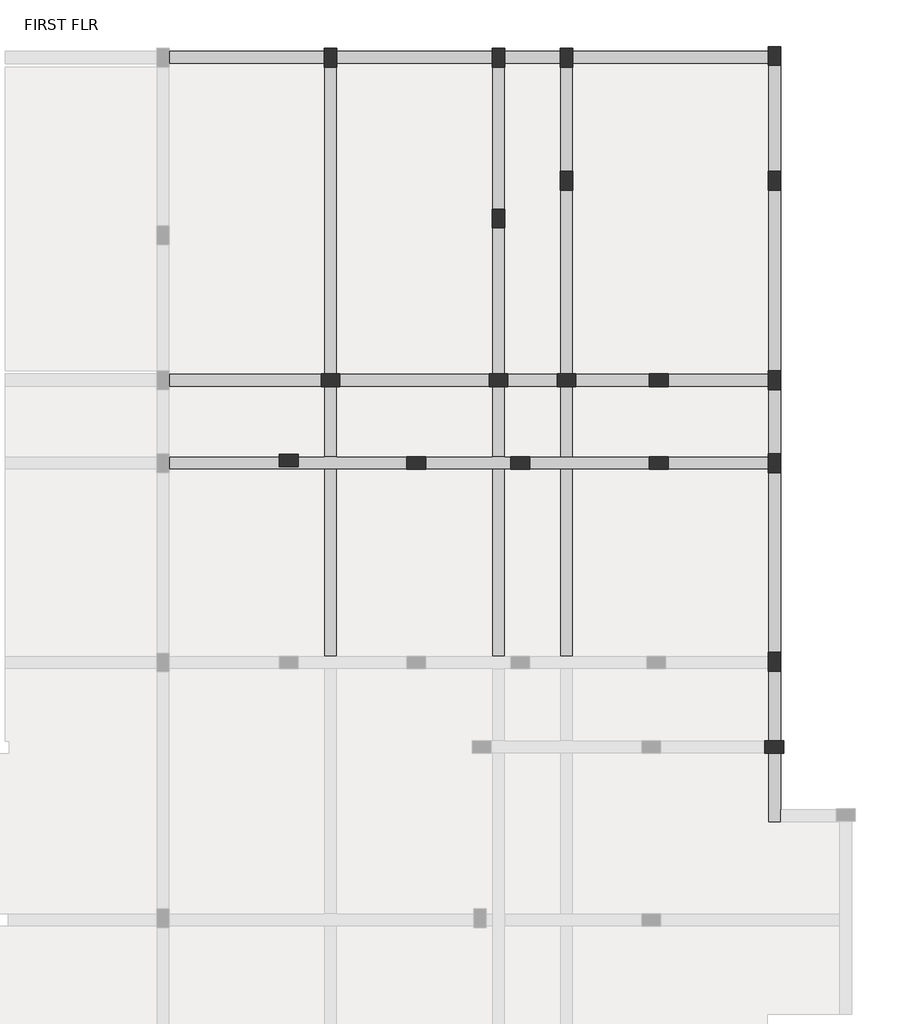
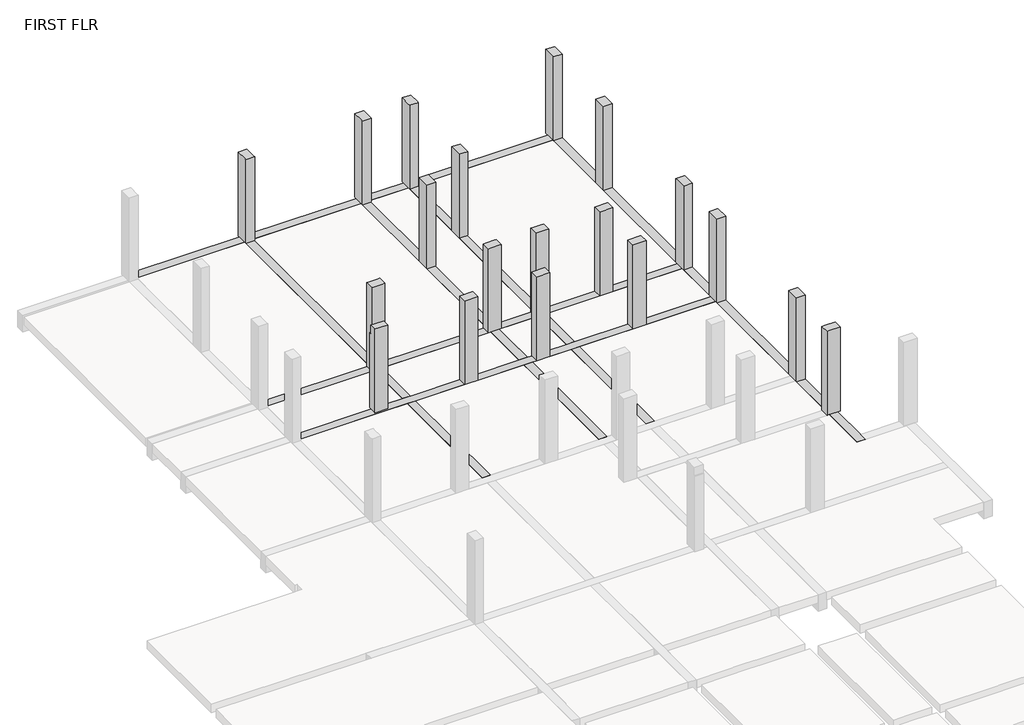
# One storey, part 5 of 5: 30 beams, 19 columns.
"""IFC4 building model written with IfcOpenShell, lengths in millimetres."""

from ifc_helpers import new_model, si_unit, frame, origin, place, context, project, spatial, polyline, outline, extrude, faceted_brep, element, save

model = new_model("IFC4")

# Units and contexts
model_context = context("Model", 3, world=origin())
ifc_project = project(units=[si_unit("LENGTHUNIT", "METRE", prefix="MILLI")], contexts=[model_context])

# Site, building, storey
site = spatial("IfcSite", under=ifc_project)
building = spatial("IfcBuilding", under=site)
storey = spatial("IfcBuildingStorey", under=building, Name="FIRST FLR", Elevation=3000.0)

# Beams
placement = place(None, origin())
element("IfcBeam", 1, ObjectType="M_Concrete-Rectangular Beam : 300 x 600mm", at=placement, inside=storey, context=model_context, shape_type="Brep", body=[
    faceted_brep([(2024.7296816, 21537.8349362, 3000.0), (2024.7296816, 21837.8349362, 3000.0), (-1671.7865686, 21837.8349362, 3000.0), (-1671.7865686, 21537.8349362, 3000.0), (2024.7296816, 21537.8349362, 2400.0), (2024.7296816, 21537.8349362, 2700.0), (-1671.7865686, 21537.8349362, 2700.0), (-1671.7865686, 21537.8349362, 2400.0), (2024.7296816, 21837.8349362, 2400.0), (-1671.7865686, 21837.8349362, 2400.0)], [[[0, 1, 2, 3]], [[4, 5, 0, 3, 6, 7]], [[8, 4, 7, 9]], [[1, 8, 9, 2]], [[2, 9, 7, 6, 3]], [[1, 0, 5, 4, 8]]]),
])
element("IfcBeam", 2, ObjectType="M_Concrete-Rectangular Beam : 300 x 600mm", at=placement, inside=storey, context=model_context, shape_type="Brep", body=[
    faceted_brep([(6032.5248054, 21537.8349362, 3000.0), (6032.5248054, 21837.8349362, 3000.0), (2324.7296816, 21837.8349362, 3000.0), (2324.7296816, 21537.8349362, 3000.0), (6032.5248054, 21537.8349362, 2400.0), (6032.5248054, 21537.8349362, 2700.0), (2324.7296816, 21537.8349362, 2700.0), (2324.7296816, 21537.8349362, 2400.0), (6032.5248054, 21837.8349362, 2400.0), (2324.7296816, 21837.8349362, 2400.0)], [[[0, 1, 2, 3]], [[4, 5, 0, 3, 6, 7]], [[8, 4, 7, 9]], [[1, 8, 9, 2]], [[2, 9, 7, 6, 3]], [[1, 0, 5, 4, 8]]]),
])
element("IfcBeam", 3, ObjectType="M_Concrete-Rectangular Beam : 300 x 600mm", at=placement, inside=storey, context=model_context, shape_type="Brep", body=[
    faceted_brep([(7656.8679014, 21537.8349362, 3000.0), (7656.8679014, 21837.8349362, 3000.0), (6332.5248054, 21837.8349362, 3000.0), (6332.5248054, 21537.8349362, 3000.0), (7656.8679014, 21537.8349362, 2400.0), (7656.8679014, 21537.8349362, 2700.0), (6332.5248054, 21537.8349362, 2700.0), (6332.5248054, 21537.8349362, 2400.0), (7656.8679014, 21837.8349362, 2400.0), (6332.5248054, 21837.8349362, 2400.0)], [[[0, 1, 2, 3]], [[4, 5, 0, 3, 6, 7]], [[8, 4, 7, 9]], [[1, 8, 9, 2]], [[2, 9, 7, 6, 3]], [[1, 0, 5, 4, 8]]]),
])
element("IfcBeam", 4, ObjectType="M_Concrete-Rectangular Beam : 300 x 600mm", at=placement, inside=storey, context=model_context, shape_type="Brep", body=[
    faceted_brep([(7956.8679014, 21837.8349362, 3000.0), (7956.8679014, 21537.8349362, 3000.0), (12619.1163908, 21537.8349362, 3000.0), (12619.1163908, 21837.8349362, 3000.0), (7956.8679014, 21537.8349362, 2700.0), (7956.8679014, 21537.8349362, 2400.0), (12619.1163908, 21537.8349362, 2400.0), (12619.1163908, 21537.8349362, 2700.0), (7956.8679014, 21837.8349362, 2400.0), (12619.1163908, 21837.8349362, 2400.0)], [[[0, 1, 2, 3]], [[1, 4, 5, 6, 7, 2]], [[5, 8, 9, 6]], [[8, 0, 3, 9]], [[0, 8, 5, 4, 1]], [[3, 2, 7, 6, 9]]]),
])
element("IfcBeam", 5, ObjectType="M_Concrete-Rectangular Beam : 300 x 600mm", at=placement, inside=storey, context=model_context, shape_type="Brep", body=[
    faceted_brep([(12916.8679014, 5087.6057249, 3000.0), (12616.8679014, 5087.6057249, 3000.0), (12616.8679014, 3435.7536525, 3000.0), (12916.8679014, 3435.7536525, 3000.0), (12916.8679014, 3735.7536525, 3000.0), (12616.8679014, 5087.6057249, 2700.0), (12616.8679014, 5087.6057249, 2400.0), (12616.8679014, 3435.7536525, 2400.0), (12616.8679014, 3435.7536525, 2700.0), (12916.8679014, 5087.6057249, 2400.0), (12916.8679014, 3735.7536525, 2400.0), (12916.8679014, 3435.7536525, 2400.0), (12916.8679014, 3435.7536525, 2700.0)], [[[0, 1, 2, 3, 4]], [[2, 1, 5, 6, 7, 8]], [[6, 9, 10, 11, 7]], [[9, 0, 4, 3, 12, 11, 10]], [[0, 9, 6, 5, 1]], [[3, 2, 8, 7, 11, 12]]]),
])
element("IfcBeam", 6, ObjectType="M_Concrete-Rectangular Beam : 300 x 600mm", at=placement, inside=storey, context=model_context, shape_type="Brep", body=[
    faceted_brep([(12616.8679014, 5387.6057249, 3000.0), (12916.8679014, 5387.6057249, 3000.0), (12916.8679014, 7044.7076276, 3000.0), (12619.1163908, 7044.7076276, 3000.0), (12619.1163908, 7399.7076276, 3000.0), (12616.8679014, 7399.7076276, 3000.0), (12616.8679014, 7099.7076276, 3000.0), (12616.8679014, 7399.7076276, 2400.0), (12616.8679014, 7099.7076276, 2400.0), (12616.8679014, 5387.6057249, 2400.0), (12616.8679014, 5387.6057249, 2700.0), (12616.8679014, 7399.7076276, 2700.0), (12916.8679014, 5387.6057249, 2400.0), (12619.1163908, 7399.7076276, 2400.0), (12619.1163908, 7044.7076276, 2400.0), (12916.8679014, 7044.7076276, 2400.0)], [[[0, 1, 2, 3, 4, 5, 6]], [[7, 8, 9, 10, 0, 6, 5, 11]], [[12, 9, 8, 7, 13, 14, 15]], [[1, 12, 15, 2]], [[1, 0, 10, 9, 12]], [[14, 3, 2, 15]], [[3, 14, 13, 4]], [[5, 4, 13, 7, 11]]]),
])
element("IfcBeam", 7, ObjectType="M_Concrete-Rectangular Beam : 300 x 600mm", at=placement, inside=storey, context=model_context, shape_type="SweptSolid", body=[
    extrude(outline(polyline([(12619.1163908, 11782.4075451), (12919.1163908, 11782.4075451), (12919.1163908, 7494.7076276), (12619.1163908, 7494.7076276), (12619.1163908, 11782.4075451)])), frame((0.0, 0.0, 2400.0), z_axis=(0.0, 0.0, 1.0), x_axis=(1.0, 0.0, 0.0)), (0.0, 0.0, 1.0), 600.0),
])
element("IfcBeam", 8, ObjectType="M_Concrete-Rectangular Beam : 300 x 600mm", at=placement, inside=storey, context=model_context, shape_type="Brep", body=[
    faceted_brep([(12619.1163908, 13762.5179708, 3000.0), (12619.1163908, 12232.4075451, 3000.0), (12919.1163908, 12232.4075451, 3000.0), (12919.1163908, 13762.5179708, 3000.0), (12919.1163908, 12232.4075451, 2400.0), (12919.1163908, 13762.5179708, 2400.0), (12619.1163908, 12232.4075451, 2400.0), (12619.1163908, 13762.5179708, 2400.0), (12619.1163908, 13762.5179708, 2700.0), (12619.1163908, 12232.4075451, 2700.0)], [[[0, 1, 2, 3]], [[3, 2, 4, 5]], [[5, 4, 6, 7]], [[1, 0, 8, 7, 6, 9]], [[0, 3, 5, 7, 8]], [[6, 4, 2, 1, 9]]]),
])
element("IfcBeam", 9, ObjectType="M_Concrete-Rectangular Beam : 300 x 600mm", at=placement, inside=storey, context=model_context, shape_type="Brep", body=[
    faceted_brep([(12619.1163908, 18524.7148651, 3000.0), (12619.1163908, 14212.5179708, 3000.0), (12919.1163908, 14212.5179708, 3000.0), (12919.1163908, 18524.7148651, 3000.0), (12919.1163908, 14212.5179708, 2400.0), (12919.1163908, 18524.7148651, 2400.0), (12619.1163908, 14212.5179708, 2400.0), (12619.1163908, 18524.7148651, 2400.0), (12619.1163908, 18524.7148651, 2700.0), (12619.1163908, 14212.5179708, 2700.0)], [[[0, 1, 2, 3]], [[3, 2, 4, 5]], [[5, 4, 6, 7]], [[1, 0, 8, 7, 6, 9]], [[0, 3, 5, 7, 8]], [[6, 4, 2, 1, 9]]]),
])
element("IfcBeam", 10, ObjectType="M_Concrete-Rectangular Beam : 300 x 600mm", at=placement, inside=storey, context=model_context, shape_type="Brep", body=[
    faceted_brep([(12619.1163908, 21502.8349362, 3000.0), (12619.1163908, 18974.7148651, 3000.0), (12919.1163908, 18974.7148651, 3000.0), (12919.1163908, 21502.8349362, 3000.0), (12919.1163908, 18974.7148651, 2400.0), (12919.1163908, 21502.8349362, 2400.0), (12619.1163908, 18974.7148651, 2400.0), (12619.1163908, 21502.8349362, 2400.0), (12619.1163908, 21502.8349362, 2700.0), (12619.1163908, 18974.7148651, 2700.0)], [[[0, 1, 2, 3]], [[3, 2, 4, 5]], [[5, 4, 6, 7]], [[1, 0, 8, 7, 6, 9]], [[6, 4, 2, 1, 9]], [[0, 3, 5, 7, 8]]]),
])
element("IfcBeam", 11, ObjectType="M_Concrete-Rectangular Beam : 300 x 600mm", at=placement, inside=storey, context=model_context, shape_type="Brep", body=[
    faceted_brep([(2324.7296816, 21462.8349362, 3000.0), (2024.7296816, 21462.8349362, 3000.0), (2024.7296816, 14137.5179708, 3000.0), (2324.7296816, 14137.5179708, 3000.0), (2024.7296816, 21462.8349362, 2700.0), (2024.7296816, 21462.8349362, 2400.0), (2024.7296816, 14137.5179708, 2400.0), (2024.7296816, 14137.5179708, 2700.0), (2324.7296816, 21462.8349362, 2400.0), (2324.7296816, 14137.5179708, 2400.0), (2324.7296816, 14137.5179708, 2700.0), (2324.7296816, 21462.8349362, 2700.0)], [[[0, 1, 2, 3]], [[2, 1, 4, 5, 6, 7]], [[5, 8, 9, 6]], [[0, 3, 10, 9, 8, 11]], [[1, 0, 11, 8, 5, 4]], [[3, 2, 7, 6, 9, 10]]]),
])
element("IfcBeam", 12, ObjectType="M_Concrete-Rectangular Beam : 300 x 600mm", at=placement, inside=storey, context=model_context, shape_type="Brep", body=[
    faceted_brep([(2324.7296816, 13837.5179708, 3000.0), (2024.7296816, 13837.5179708, 3000.0), (2024.7296816, 12157.4075451, 3000.0), (2324.7296816, 12157.4075451, 3000.0), (2024.7296816, 13837.5179708, 2700.0), (2024.7296816, 13837.5179708, 2400.0), (2024.7296816, 12157.4075451, 2400.0), (2024.7296816, 12157.4075451, 2700.0), (2324.7296816, 13837.5179708, 2400.0), (2324.7296816, 12157.4075451, 2400.0), (2324.7296816, 12157.4075451, 2700.0), (2324.7296816, 13837.5179708, 2700.0)], [[[0, 1, 2, 3]], [[2, 1, 4, 5, 6, 7]], [[5, 8, 9, 6]], [[0, 3, 10, 9, 8, 11]], [[1, 0, 11, 8, 5, 4]], [[3, 2, 7, 6, 9, 10]]]),
])
element("IfcBeam", 13, ObjectType="M_Concrete-Rectangular Beam : 300 x 600mm", at=placement, inside=storey, context=model_context, shape_type="Brep", body=[
    faceted_brep([(6332.5248054, 21462.8349362, 3000.0), (6032.5248054, 21462.8349362, 3000.0), (6032.5248054, 18074.7148651, 3000.0), (6332.5248054, 18074.7148651, 3000.0), (6032.5248054, 21462.8349362, 2700.0), (6032.5248054, 21462.8349362, 2400.0), (6032.5248054, 18074.7148651, 2400.0), (6032.5248054, 18074.7148651, 2700.0), (6332.5248054, 21462.8349362, 2400.0), (6332.5248054, 18074.7148651, 2400.0), (6332.5248054, 18074.7148651, 2700.0), (6332.5248054, 21462.8349362, 2700.0)], [[[0, 1, 2, 3]], [[2, 1, 4, 5, 6, 7]], [[5, 8, 9, 6]], [[0, 3, 10, 9, 8, 11]], [[1, 0, 11, 8, 5, 4]], [[3, 2, 7, 6, 9, 10]]]),
])
element("IfcBeam", 14, ObjectType="M_Concrete-Rectangular Beam : 300 x 600mm", at=placement, inside=storey, context=model_context, shape_type="Brep", body=[
    faceted_brep([(6332.5248054, 17624.7148651, 3000.0), (6032.5248054, 17624.7148651, 3000.0), (6032.5248054, 14137.5179708, 3000.0), (6332.5248054, 14137.5179708, 3000.0), (6032.5248054, 17624.7148651, 2700.0), (6032.5248054, 17624.7148651, 2400.0), (6032.5248054, 14137.5179708, 2400.0), (6032.5248054, 14137.5179708, 2700.0), (6332.5248054, 17624.7148651, 2400.0), (6332.5248054, 14137.5179708, 2400.0), (6332.5248054, 14137.5179708, 2700.0), (6332.5248054, 17624.7148651, 2700.0)], [[[0, 1, 2, 3]], [[2, 1, 4, 5, 6, 7]], [[5, 8, 9, 6]], [[0, 3, 10, 9, 8, 11]], [[1, 0, 11, 8, 5, 4]], [[3, 2, 7, 6, 9, 10]]]),
])
element("IfcBeam", 15, ObjectType="M_Concrete-Rectangular Beam : 300 x 600mm", at=placement, inside=storey, context=model_context, shape_type="Brep", body=[
    faceted_brep([(6332.5248054, 13837.5179708, 3000.0), (6032.5248054, 13837.5179708, 3000.0), (6032.5248054, 12157.4075451, 3000.0), (6332.5248054, 12157.4075451, 3000.0), (6032.5248054, 13837.5179708, 2700.0), (6032.5248054, 13837.5179708, 2400.0), (6032.5248054, 12157.4075451, 2400.0), (6032.5248054, 12157.4075451, 2700.0), (6332.5248054, 13837.5179708, 2400.0), (6332.5248054, 12157.4075451, 2400.0), (6332.5248054, 12157.4075451, 2700.0), (6332.5248054, 13837.5179708, 2700.0)], [[[0, 1, 2, 3]], [[2, 1, 4, 5, 6, 7]], [[5, 8, 9, 6]], [[0, 3, 10, 9, 8, 11]], [[1, 0, 11, 8, 5, 4]], [[3, 2, 7, 6, 9, 10]]]),
])
element("IfcBeam", 16, ObjectType="M_Concrete-Rectangular Beam : 300 x 600mm", at=placement, inside=storey, context=model_context, shape_type="Brep", body=[
    faceted_brep([(7956.8679014, 21462.8349362, 3000.0), (7656.8679014, 21462.8349362, 3000.0), (7656.8679014, 18974.7148651, 3000.0), (7956.8679014, 18974.7148651, 3000.0), (7656.8679014, 21462.8349362, 2700.0), (7656.8679014, 21462.8349362, 2400.0), (7656.8679014, 18974.7148651, 2400.0), (7656.8679014, 18974.7148651, 2700.0), (7956.8679014, 21462.8349362, 2400.0), (7956.8679014, 18974.7148651, 2400.0), (7956.8679014, 18974.7148651, 2700.0), (7956.8679014, 21462.8349362, 2700.0)], [[[0, 1, 2, 3]], [[2, 1, 4, 5, 6, 7]], [[5, 8, 9, 6]], [[0, 3, 10, 9, 8, 11]], [[1, 0, 11, 8, 5, 4]], [[3, 2, 7, 6, 9, 10]]]),
])
element("IfcBeam", 17, ObjectType="M_Concrete-Rectangular Beam : 300 x 600mm", at=placement, inside=storey, context=model_context, shape_type="Brep", body=[
    faceted_brep([(7956.8679014, 18524.7148651, 3000.0), (7656.8679014, 18524.7148651, 3000.0), (7656.8679014, 14137.5179708, 3000.0), (7956.8679014, 14137.5179708, 3000.0), (7656.8679014, 18524.7148651, 2700.0), (7656.8679014, 18524.7148651, 2400.0), (7656.8679014, 14137.5179708, 2400.0), (7656.8679014, 14137.5179708, 2700.0), (7956.8679014, 18524.7148651, 2400.0), (7956.8679014, 14137.5179708, 2400.0), (7956.8679014, 14137.5179708, 2700.0), (7956.8679014, 18524.7148651, 2700.0)], [[[0, 1, 2, 3]], [[2, 1, 4, 5, 6, 7]], [[5, 8, 9, 6]], [[0, 3, 10, 9, 8, 11]], [[1, 0, 11, 8, 5, 4]], [[3, 2, 7, 6, 9, 10]]]),
])
element("IfcBeam", 18, ObjectType="M_Concrete-Rectangular Beam : 300 x 600mm", at=placement, inside=storey, context=model_context, shape_type="Brep", body=[
    faceted_brep([(7956.8679014, 13837.5179708, 3000.0), (7656.8679014, 13837.5179708, 3000.0), (7656.8679014, 12157.4075451, 3000.0), (7956.8679014, 12157.4075451, 3000.0), (7656.8679014, 13837.5179708, 2700.0), (7656.8679014, 13837.5179708, 2400.0), (7656.8679014, 12157.4075451, 2400.0), (7656.8679014, 12157.4075451, 2700.0), (7956.8679014, 13837.5179708, 2400.0), (7956.8679014, 12157.4075451, 2400.0), (7956.8679014, 12157.4075451, 2700.0), (7956.8679014, 13837.5179708, 2700.0)], [[[0, 1, 2, 3]], [[2, 1, 4, 5, 6, 7]], [[5, 8, 9, 6]], [[0, 3, 10, 9, 8, 11]], [[1, 0, 11, 8, 5, 4]], [[3, 2, 7, 6, 9, 10]]]),
])
element("IfcBeam", 19, ObjectType="M_Concrete-Rectangular Beam : 300 x 600mm", at=placement, inside=storey, context=model_context, shape_type="Brep", body=[
    faceted_brep([(-1671.7865686, 14137.5179708, 3000.0), (-1671.7865686, 13837.5179708, 3000.0), (1949.7296816, 13837.5179708, 3000.0), (1949.7296816, 14137.5179708, 3000.0), (-1671.7865686, 13837.5179708, 2700.0), (-1671.7865686, 13837.5179708, 2400.0), (1949.7296816, 13837.5179708, 2400.0), (1949.7296816, 13837.5179708, 2700.0), (-1671.7865686, 14137.5179708, 2400.0), (1949.7296816, 14137.5179708, 2400.0), (1949.7296816, 14137.5179708, 2700.0), (-1671.7865686, 14137.5179708, 2700.0)], [[[0, 1, 2, 3]], [[2, 1, 4, 5, 6, 7]], [[5, 8, 9, 6]], [[0, 3, 10, 9, 8, 11]], [[1, 0, 11, 8, 5, 4]], [[3, 2, 7, 6, 9, 10]]]),
])
element("IfcBeam", 20, ObjectType="M_Concrete-Rectangular Beam : 300 x 600mm", at=placement, inside=storey, context=model_context, shape_type="Brep", body=[
    faceted_brep([(2399.7296816, 14137.5179708, 3000.0), (2399.7296816, 13837.5179708, 3000.0), (5957.5248054, 13837.5179708, 3000.0), (5957.5248054, 14137.5179708, 3000.0), (2399.7296816, 13837.5179708, 2700.0), (2399.7296816, 13837.5179708, 2400.0), (5957.5248054, 13837.5179708, 2400.0), (5957.5248054, 13837.5179708, 2700.0), (2399.7296816, 14137.5179708, 2400.0), (5957.5248054, 14137.5179708, 2400.0), (5957.5248054, 14137.5179708, 2700.0), (2399.7296816, 14137.5179708, 2700.0)], [[[0, 1, 2, 3]], [[2, 1, 4, 5, 6, 7]], [[5, 8, 9, 6]], [[0, 3, 10, 9, 8, 11]], [[1, 0, 11, 8, 5, 4]], [[3, 2, 7, 6, 9, 10]]]),
])
element("IfcBeam", 21, ObjectType="M_Concrete-Rectangular Beam : 300 x 600mm", at=placement, inside=storey, context=model_context, shape_type="Brep", body=[
    faceted_brep([(6407.5248054, 14137.5179708, 3000.0), (6407.5248054, 13837.5179708, 3000.0), (7581.8679014, 13837.5179708, 3000.0), (7581.8679014, 14137.5179708, 3000.0), (6407.5248054, 13837.5179708, 2700.0), (6407.5248054, 13837.5179708, 2400.0), (7581.8679014, 13837.5179708, 2400.0), (7581.8679014, 13837.5179708, 2700.0), (6407.5248054, 14137.5179708, 2400.0), (7581.8679014, 14137.5179708, 2400.0), (7581.8679014, 14137.5179708, 2700.0), (6407.5248054, 14137.5179708, 2700.0)], [[[0, 1, 2, 3]], [[2, 1, 4, 5, 6, 7]], [[5, 8, 9, 6]], [[0, 3, 10, 9, 8, 11]], [[1, 0, 11, 8, 5, 4]], [[3, 2, 7, 6, 9, 10]]]),
])
element("IfcBeam", 22, ObjectType="M_Concrete-Rectangular Beam : 300 x 600mm", at=placement, inside=storey, context=model_context, shape_type="Brep", body=[
    faceted_brep([(8031.8679014, 14137.5179708, 3000.0), (8031.8679014, 13837.5179708, 3000.0), (9781.8679014, 13837.5179708, 3000.0), (9781.8679014, 14137.5179708, 3000.0), (8031.8679014, 13837.5179708, 2700.0), (8031.8679014, 13837.5179708, 2400.0), (9781.8679014, 13837.5179708, 2400.0), (9781.8679014, 13837.5179708, 2700.0), (8031.8679014, 14137.5179708, 2400.0), (9781.8679014, 14137.5179708, 2400.0), (9781.8679014, 14137.5179708, 2700.0), (8031.8679014, 14137.5179708, 2700.0)], [[[0, 1, 2, 3]], [[2, 1, 4, 5, 6, 7]], [[5, 8, 9, 6]], [[0, 3, 10, 9, 8, 11]], [[1, 0, 11, 8, 5, 4]], [[3, 2, 7, 6, 9, 10]]]),
])
element("IfcBeam", 23, ObjectType="M_Concrete-Rectangular Beam : 300 x 600mm", at=placement, inside=storey, context=model_context, shape_type="Brep", body=[
    faceted_brep([(10231.8679014, 14137.5179708, 3000.0), (10231.8679014, 13837.5179708, 3000.0), (12619.1163908, 13837.5179708, 3000.0), (12619.1163908, 14137.5179708, 3000.0), (10231.8679014, 13837.5179708, 2700.0), (10231.8679014, 13837.5179708, 2400.0), (12619.1163908, 13837.5179708, 2400.0), (12619.1163908, 13837.5179708, 2700.0), (10231.8679014, 14137.5179708, 2400.0), (12619.1163908, 14137.5179708, 2400.0), (12619.1163908, 14137.5179708, 2700.0), (10231.8679014, 14137.5179708, 2700.0)], [[[0, 1, 2, 3]], [[2, 1, 4, 5, 6, 7]], [[5, 8, 9, 6]], [[0, 3, 10, 9, 8, 11]], [[1, 0, 11, 8, 5, 4]], [[3, 2, 7, 6, 9, 10]]]),
])
element("IfcBeam", 24, ObjectType="M_Concrete-Rectangular Beam : 300 x 600mm", at=placement, inside=storey, context=model_context, shape_type="Brep", body=[
    faceted_brep([(-1671.7865686, 12157.4075451, 3000.0), (-1671.7865686, 11857.4075451, 3000.0), (2024.7296816, 11857.4075451, 3000.0), (2324.7296816, 11857.4075451, 3000.0), (3997.5248054, 11857.4075451, 3000.0), (3997.5248054, 12157.4075451, 3000.0), (2324.7296816, 12157.4075451, 3000.0), (2024.7296816, 12157.4075451, 3000.0), (1399.7296816, 12157.4075451, 3000.0), (1399.7296816, 11917.4075451, 3000.0), (949.7296816, 11917.4075451, 3000.0), (949.7296816, 12157.4075451, 3000.0), (-1671.7865686, 11857.4075451, 2400.0), (2024.7296816, 11857.4075451, 2400.0), (2324.7296816, 11857.4075451, 2400.0), (3997.5248054, 11857.4075451, 2400.0), (3997.5248054, 11857.4075451, 2700.0), (-1671.7865686, 11857.4075451, 2700.0), (-1671.7865686, 12157.4075451, 2400.0), (949.7296816, 12157.4075451, 2400.0), (949.7296816, 11917.4075451, 2400.0), (1399.7296816, 11917.4075451, 2400.0), (1399.7296816, 12157.4075451, 2400.0), (2024.7296816, 12157.4075451, 2400.0), (2324.7296816, 12157.4075451, 2400.0), (3997.5248054, 12157.4075451, 2400.0), (949.7296816, 12157.4075451, 2700.0), (-1671.7865686, 12157.4075451, 2700.0), (3997.5248054, 12157.4075451, 2700.0), (1399.7296816, 12157.4075451, 2700.0)], [[[0, 1, 2, 3, 4, 5, 6, 7, 8, 9, 10, 11]], [[12, 13, 14, 15, 16, 4, 3, 2, 1, 17]], [[12, 18, 19, 20, 21, 22, 23, 24, 25, 15, 14, 13]], [[0, 11, 26, 19, 18, 27]], [[1, 0, 27, 18, 12, 17]], [[5, 4, 16, 15, 25, 28]], [[20, 10, 9, 21]], [[10, 20, 19, 26, 11]], [[21, 9, 8, 29, 22]], [[25, 24, 23, 22, 29, 8, 7, 6, 5, 28]]]),
])
element("IfcBeam", 25, ObjectType="M_Concrete-Rectangular Beam : 300 x 600mm", at=placement, inside=storey, context=model_context, shape_type="Brep", body=[
    faceted_brep([(4447.5248054, 12157.4075451, 3000.0), (4447.5248054, 11857.4075451, 3000.0), (6032.5248054, 11857.4075451, 3000.0), (6332.5248054, 11857.4075451, 3000.0), (6481.8679014, 11857.4075451, 3000.0), (6481.8679014, 12157.4075451, 3000.0), (6332.5248054, 12157.4075451, 3000.0), (6032.5248054, 12157.4075451, 3000.0), (4447.5248054, 11857.4075451, 2400.0), (6032.5248054, 11857.4075451, 2400.0), (6332.5248054, 11857.4075451, 2400.0), (6481.8679014, 11857.4075451, 2400.0), (6481.8679014, 11857.4075451, 2700.0), (4447.5248054, 11857.4075451, 2700.0), (4447.5248054, 12157.4075451, 2400.0), (6032.5248054, 12157.4075451, 2400.0), (6332.5248054, 12157.4075451, 2400.0), (6481.8679014, 12157.4075451, 2400.0), (4447.5248054, 12157.4075451, 2700.0), (6481.8679014, 12157.4075451, 2700.0)], [[[0, 1, 2, 3, 4, 5, 6, 7]], [[8, 9, 10, 11, 12, 4, 3, 2, 1, 13]], [[8, 14, 15, 16, 17, 11, 10, 9]], [[17, 16, 15, 14, 18, 0, 7, 6, 5, 19]], [[1, 0, 18, 14, 8, 13]], [[5, 4, 12, 11, 17, 19]]]),
])
element("IfcBeam", 26, ObjectType="M_Concrete-Rectangular Beam : 300 x 600mm", at=placement, inside=storey, context=model_context, shape_type="Brep", body=[
    faceted_brep([(6931.8679014, 12157.4075451, 3000.0), (6931.8679014, 11857.4075451, 3000.0), (7656.8679014, 11857.4075451, 3000.0), (7956.8679014, 11857.4075451, 3000.0), (9781.8679014, 11857.4075451, 3000.0), (9781.8679014, 12157.4075451, 3000.0), (7956.8679014, 12157.4075451, 3000.0), (7656.8679014, 12157.4075451, 3000.0), (6931.8679014, 11857.4075451, 2400.0), (7656.8679014, 11857.4075451, 2400.0), (7956.8679014, 11857.4075451, 2400.0), (9781.8679014, 11857.4075451, 2400.0), (9781.8679014, 11857.4075451, 2700.0), (6931.8679014, 11857.4075451, 2700.0), (6931.8679014, 12157.4075451, 2400.0), (7656.8679014, 12157.4075451, 2400.0), (7956.8679014, 12157.4075451, 2400.0), (9781.8679014, 12157.4075451, 2400.0), (6931.8679014, 12157.4075451, 2700.0), (9781.8679014, 12157.4075451, 2700.0)], [[[0, 1, 2, 3, 4, 5, 6, 7]], [[8, 9, 10, 11, 12, 4, 3, 2, 1, 13]], [[8, 14, 15, 16, 17, 11, 10, 9]], [[17, 16, 15, 14, 18, 0, 7, 6, 5, 19]], [[1, 0, 18, 14, 8, 13]], [[5, 4, 12, 11, 17, 19]]]),
])
element("IfcBeam", 27, ObjectType="M_Concrete-Rectangular Beam : 300 x 600mm", at=placement, inside=storey, context=model_context, shape_type="Brep", body=[
    faceted_brep([(10231.8679014, 12157.4075451, 3000.0), (10231.8679014, 11857.4075451, 3000.0), (12616.8679014, 11857.4075451, 3000.0), (12619.1163908, 11857.4075451, 3000.0), (12619.1163908, 12157.4075451, 3000.0), (10231.8679014, 11857.4075451, 2400.0), (12619.1163908, 11857.4075451, 2400.0), (10231.8679014, 11857.4075451, 2700.0), (10231.8679014, 12157.4075451, 2400.0), (12619.1163908, 12157.4075451, 2400.0), (12619.1163908, 12157.4075451, 2700.0), (10231.8679014, 12157.4075451, 2700.0)], [[[0, 1, 2, 3, 4]], [[5, 6, 3, 2, 1, 7]], [[5, 8, 9, 6]], [[0, 4, 10, 9, 8, 11]], [[1, 0, 11, 8, 5, 7]], [[4, 3, 6, 9, 10]]]),
])
element("IfcBeam", 28, ObjectType="M_Concrete-Rectangular Beam : 300 x 600mm", at=placement, inside=storey, context=model_context, shape_type="Brep", body=[
    faceted_brep([(2324.7296816, 11857.4075451, 3000.0), (2024.7296816, 11857.4075451, 3000.0), (2024.7296816, 7399.7076276, 3000.0), (2324.7296816, 7399.7076276, 3000.0), (2024.7296816, 11857.4075451, 2700.0), (2024.7296816, 11857.4075451, 2400.0), (2024.7296816, 7399.7076276, 2400.0), (2024.7296816, 7399.7076276, 2700.0), (2324.7296816, 11857.4075451, 2400.0), (2324.7296816, 7399.7076276, 2400.0), (2324.7296816, 7399.7076276, 2700.0), (2324.7296816, 11857.4075451, 2700.0)], [[[0, 1, 2, 3]], [[2, 1, 4, 5, 6, 7]], [[5, 8, 9, 6]], [[0, 3, 10, 9, 8, 11]], [[1, 0, 11, 8, 5, 4]], [[3, 2, 7, 6, 9, 10]]]),
])
element("IfcBeam", 29, ObjectType="M_Concrete-Rectangular Beam : 300 x 600mm", at=placement, inside=storey, context=model_context, shape_type="Brep", body=[
    faceted_brep([(6332.5248054, 11857.4075451, 3000.0), (6032.5248054, 11857.4075451, 3000.0), (6032.5248054, 7399.7076276, 3000.0), (6332.5248054, 7399.7076276, 3000.0), (6032.5248054, 11857.4075451, 2700.0), (6032.5248054, 11857.4075451, 2400.0), (6032.5248054, 7399.7076276, 2400.0), (6032.5248054, 7399.7076276, 2700.0), (6332.5248054, 11857.4075451, 2400.0), (6332.5248054, 7399.7076276, 2400.0), (6332.5248054, 7399.7076276, 2700.0), (6332.5248054, 11857.4075451, 2700.0)], [[[0, 1, 2, 3]], [[2, 1, 4, 5, 6, 7]], [[5, 8, 9, 6]], [[0, 3, 10, 9, 8, 11]], [[1, 0, 11, 8, 5, 4]], [[3, 2, 7, 6, 9, 10]]]),
])
element("IfcBeam", 30, ObjectType="M_Concrete-Rectangular Beam : 300 x 600mm", at=placement, inside=storey, context=model_context, shape_type="Brep", body=[
    faceted_brep([(7956.8679014, 11857.4075451, 3000.0), (7656.8679014, 11857.4075451, 3000.0), (7656.8679014, 7399.7076276, 3000.0), (7956.8679014, 7399.7076276, 3000.0), (7656.8679014, 11857.4075451, 2700.0), (7656.8679014, 11857.4075451, 2400.0), (7656.8679014, 7399.7076276, 2400.0), (7656.8679014, 7399.7076276, 2700.0), (7956.8679014, 11857.4075451, 2400.0), (7956.8679014, 7399.7076276, 2400.0), (7956.8679014, 7399.7076276, 2700.0), (7956.8679014, 11857.4075451, 2700.0)], [[[0, 1, 2, 3]], [[2, 1, 4, 5, 6, 7]], [[5, 8, 9, 6]], [[0, 3, 10, 9, 8, 11]], [[1, 0, 11, 8, 5, 4]], [[3, 2, 7, 6, 9, 10]]]),
])

# Columns
element("IfcColumn", 31, ObjectType="M_Concrete-Rectangular-Column : 300 x 450mm", at=placement, inside=storey, context=model_context, shape_type="Brep", body=[
    faceted_brep([(2324.7296816, 21912.8349362, 3000.0), (2324.7296816, 21462.8349362, 3000.0), (2024.7296816, 21462.8349362, 3000.0), (2024.7296816, 21912.8349362, 3000.0), (2324.7296816, 21912.8349362, 6048.0), (2324.7296816, 21537.8349362, 6048.0), (2324.7296816, 21462.8349362, 6048.0), (2324.7296816, 21462.8349362, 5748.0), (2024.7296816, 21462.8349362, 6048.0), (2024.7296816, 21462.8349362, 5748.0), (2024.7296816, 21537.8349362, 6048.0), (2024.7296816, 21912.8349362, 6048.0)], [[[0, 1, 2, 3]], [[1, 0, 4, 5, 6, 7]], [[2, 1, 7, 6, 8, 9]], [[3, 2, 9, 8, 10, 11]], [[0, 3, 11, 4]], [[8, 6, 5, 4, 11, 10]]]),
])
element("IfcColumn", 32, ObjectType="M_Concrete-Rectangular-Column : 300 x 450mm", at=placement, inside=storey, context=model_context, shape_type="Brep", body=[
    faceted_brep([(6332.5248054, 21912.8349362, 3000.0), (6332.5248054, 21462.8349362, 3000.0), (6032.5248054, 21462.8349362, 3000.0), (6032.5248054, 21912.8349362, 3000.0), (6332.5248054, 21912.8349362, 6048.0), (6332.5248054, 21537.8349362, 6048.0), (6332.5248054, 21462.8349362, 6048.0), (6332.5248054, 21462.8349362, 5748.0), (6032.5248054, 21462.8349362, 6048.0), (6032.5248054, 21462.8349362, 5748.0), (6032.5248054, 21537.8349362, 6048.0), (6032.5248054, 21912.8349362, 6048.0)], [[[0, 1, 2, 3]], [[1, 0, 4, 5, 6, 7]], [[2, 1, 7, 6, 8, 9]], [[3, 2, 9, 8, 10, 11]], [[0, 3, 11, 4]], [[8, 6, 5, 4, 11, 10]]]),
])
element("IfcColumn", 33, ObjectType="M_Concrete-Rectangular-Column : 300 x 450mm", at=placement, inside=storey, context=model_context, shape_type="Brep", body=[
    faceted_brep([(7956.8679014, 21912.8349362, 3000.0), (7956.8679014, 21462.8349362, 3000.0), (7656.8679014, 21462.8349362, 3000.0), (7656.8679014, 21912.8349362, 3000.0), (7956.8679014, 21912.8349362, 6048.0), (7956.8679014, 21537.8349362, 6048.0), (7956.8679014, 21462.8349362, 6048.0), (7956.8679014, 21462.8349362, 5748.0), (7656.8679014, 21462.8349362, 6048.0), (7656.8679014, 21462.8349362, 5748.0), (7656.8679014, 21537.8349362, 6048.0), (7656.8679014, 21912.8349362, 6048.0)], [[[0, 1, 2, 3]], [[1, 0, 4, 5, 6, 7]], [[2, 1, 7, 6, 8, 9]], [[3, 2, 9, 8, 10, 11]], [[0, 3, 11, 4]], [[8, 6, 5, 4, 11, 10]]]),
])
element("IfcColumn", 34, ObjectType="M_Concrete-Rectangular-Column : 300 x 450mm", at=placement, inside=storey, context=model_context, shape_type="Brep", body=[
    faceted_brep([(12919.1163908, 21952.8349362, 3000.0), (12919.1163908, 21502.8349362, 3000.0), (12619.1163908, 21502.8349362, 3000.0), (12619.1163908, 21952.8349362, 3000.0), (12919.1163908, 21952.8349362, 6048.0), (12919.1163908, 21502.8349362, 6048.0), (12619.1163908, 21502.8349362, 6048.0), (12619.1163908, 21502.8349362, 5748.0), (12619.1163908, 21537.8349362, 6048.0), (12619.1163908, 21952.8349362, 6048.0)], [[[0, 1, 2, 3]], [[1, 0, 4, 5]], [[2, 1, 5, 6, 7]], [[3, 2, 7, 6, 8, 9]], [[0, 3, 9, 4]], [[5, 4, 9, 8, 6]]]),
])
element("IfcColumn", 35, ObjectType="M_Concrete-Rectangular-Column : 300 x 450mm", at=placement, inside=storey, context=model_context, shape_type="Brep", body=[
    faceted_brep([(12919.1163908, 18974.7148651, 3000.0), (12919.1163908, 18524.7148651, 3000.0), (12619.1163908, 18524.7148651, 3000.0), (12619.1163908, 18974.7148651, 3000.0), (12919.1163908, 18974.7148651, 6048.0), (12919.1163908, 18524.7148651, 6048.0), (12619.1163908, 18524.7148651, 6048.0), (12619.1163908, 18524.7148651, 5748.0), (12619.1163908, 18974.7148651, 6048.0), (12619.1163908, 18974.7148651, 5748.0)], [[[0, 1, 2, 3]], [[1, 0, 4, 5]], [[2, 1, 5, 6, 7]], [[3, 2, 7, 6, 8, 9]], [[0, 3, 9, 8, 4]], [[5, 4, 8, 6]]]),
])
element("IfcColumn", 36, ObjectType="M_Concrete-Rectangular-Column : 300 x 450mm", at=placement, inside=storey, context=model_context, shape_type="Brep", body=[
    faceted_brep([(7956.8679014, 18974.7148651, 3000.0), (7956.8679014, 18524.7148651, 3000.0), (7656.8679014, 18524.7148651, 3000.0), (7656.8679014, 18974.7148651, 3000.0), (7956.8679014, 18974.7148651, 5748.0), (7956.8679014, 18974.7148651, 6048.0), (7956.8679014, 18524.7148651, 6048.0), (7956.8679014, 18524.7148651, 5748.0), (7656.8679014, 18524.7148651, 6048.0), (7656.8679014, 18524.7148651, 5748.0), (7656.8679014, 18974.7148651, 6048.0), (7656.8679014, 18974.7148651, 5748.0)], [[[0, 1, 2, 3]], [[1, 0, 4, 5, 6, 7]], [[2, 1, 7, 6, 8, 9]], [[3, 2, 9, 8, 10, 11]], [[0, 3, 11, 10, 5, 4]], [[6, 5, 10, 8]]]),
])
element("IfcColumn", 37, ObjectType="M_Concrete-Rectangular-Column : 300 x 450mm", at=placement, inside=storey, context=model_context, shape_type="Brep", body=[
    faceted_brep([(6332.5248054, 18074.7148651, 3000.0), (6332.5248054, 17624.7148651, 3000.0), (6032.5248054, 17624.7148651, 3000.0), (6032.5248054, 18074.7148651, 3000.0), (6332.5248054, 18074.7148651, 5748.0), (6332.5248054, 18074.7148651, 6048.0), (6332.5248054, 17624.7148651, 6048.0), (6332.5248054, 17624.7148651, 5748.0), (6032.5248054, 17624.7148651, 6048.0), (6032.5248054, 17624.7148651, 5748.0), (6032.5248054, 18074.7148651, 6048.0), (6032.5248054, 18074.7148651, 5748.0)], [[[0, 1, 2, 3]], [[1, 0, 4, 5, 6, 7]], [[2, 1, 7, 6, 8, 9]], [[3, 2, 9, 8, 10, 11]], [[0, 3, 11, 10, 5, 4]], [[6, 5, 10, 8]]]),
])
element("IfcColumn", 38, ObjectType="M_Concrete-Rectangular-Column : 300 x 450mm", at=placement, inside=storey, context=model_context, shape_type="Brep", body=[
    faceted_brep([(1949.7296816, 14137.5179708, 3000.0), (2399.7296816, 14137.5179708, 3000.0), (2399.7296816, 13837.5179708, 3000.0), (1949.7296816, 13837.5179708, 3000.0), (1949.7296816, 14137.5179708, 5748.0), (1949.7296816, 14137.5179708, 6048.0), (2024.7296816, 14137.5179708, 6048.0), (2324.7296816, 14137.5179708, 6048.0), (2399.7296816, 14137.5179708, 6048.0), (2399.7296816, 14137.5179708, 5748.0), (2399.7296816, 13837.5179708, 6048.0), (2399.7296816, 13837.5179708, 5748.0), (2324.7296816, 13837.5179708, 6048.0), (2024.7296816, 13837.5179708, 6048.0), (1949.7296816, 13837.5179708, 6048.0), (1949.7296816, 13837.5179708, 5748.0)], [[[0, 1, 2, 3]], [[1, 0, 4, 5, 6, 7, 8, 9]], [[2, 1, 9, 8, 10, 11]], [[3, 2, 11, 10, 12, 13, 14, 15]], [[0, 3, 15, 14, 5, 4]], [[10, 8, 7, 6, 5, 14, 13, 12]]]),
])
element("IfcColumn", 39, ObjectType="M_Concrete-Rectangular-Column : 300 x 450mm", at=placement, inside=storey, context=model_context, shape_type="Brep", body=[
    faceted_brep([(5957.5248054, 14137.5179708, 3000.0), (6407.5248054, 14137.5179708, 3000.0), (6407.5248054, 13837.5179708, 3000.0), (5957.5248054, 13837.5179708, 3000.0), (5957.5248054, 14137.5179708, 5748.0), (5957.5248054, 14137.5179708, 6048.0), (6032.5248054, 14137.5179708, 6048.0), (6332.5248054, 14137.5179708, 6048.0), (6407.5248054, 14137.5179708, 6048.0), (6407.5248054, 14137.5179708, 5748.0), (6407.5248054, 13837.5179708, 6048.0), (6407.5248054, 13837.5179708, 5748.0), (6332.5248054, 13837.5179708, 6048.0), (6032.5248054, 13837.5179708, 6048.0), (5957.5248054, 13837.5179708, 6048.0), (5957.5248054, 13837.5179708, 5748.0)], [[[0, 1, 2, 3]], [[1, 0, 4, 5, 6, 7, 8, 9]], [[2, 1, 9, 8, 10, 11]], [[3, 2, 11, 10, 12, 13, 14, 15]], [[0, 3, 15, 14, 5, 4]], [[10, 8, 7, 6, 5, 14, 13, 12]]]),
])
element("IfcColumn", 40, ObjectType="M_Concrete-Rectangular-Column : 300 x 450mm", at=placement, inside=storey, context=model_context, shape_type="Brep", body=[
    faceted_brep([(7581.8679014, 14137.5179708, 3000.0), (8031.8679014, 14137.5179708, 3000.0), (8031.8679014, 13837.5179708, 3000.0), (7581.8679014, 13837.5179708, 3000.0), (7581.8679014, 14137.5179708, 5748.0), (7581.8679014, 14137.5179708, 6048.0), (7656.8679014, 14137.5179708, 6048.0), (7956.8679014, 14137.5179708, 6048.0), (8031.8679014, 14137.5179708, 6048.0), (8031.8679014, 14137.5179708, 5748.0), (8031.8679014, 13837.5179708, 6048.0), (8031.8679014, 13837.5179708, 5748.0), (7956.8679014, 13837.5179708, 6048.0), (7656.8679014, 13837.5179708, 6048.0), (7581.8679014, 13837.5179708, 6048.0), (7581.8679014, 13837.5179708, 5748.0)], [[[0, 1, 2, 3]], [[1, 0, 4, 5, 6, 7, 8, 9]], [[2, 1, 9, 8, 10, 11]], [[3, 2, 11, 10, 12, 13, 14, 15]], [[0, 3, 15, 14, 5, 4]], [[10, 8, 7, 6, 5, 14, 13, 12]]]),
])
element("IfcColumn", 41, ObjectType="M_Concrete-Rectangular-Column : 300 x 450mm", at=placement, inside=storey, context=model_context, shape_type="Brep", body=[
    faceted_brep([(9781.8679014, 14137.5179708, 3000.0), (10231.8679014, 14137.5179708, 3000.0), (10231.8679014, 13837.5179708, 3000.0), (9781.8679014, 13837.5179708, 3000.0), (9781.8679014, 14137.5179708, 5748.0), (9781.8679014, 14137.5179708, 6048.0), (10231.8679014, 14137.5179708, 6048.0), (10231.8679014, 14137.5179708, 5748.0), (10231.8679014, 13837.5179708, 6048.0), (10231.8679014, 13837.5179708, 5748.0), (9781.8679014, 13837.5179708, 6048.0), (9781.8679014, 13837.5179708, 5748.0)], [[[0, 1, 2, 3]], [[1, 0, 4, 5, 6, 7]], [[2, 1, 7, 6, 8, 9]], [[3, 2, 9, 8, 10, 11]], [[0, 3, 11, 10, 5, 4]], [[6, 5, 10, 8]]]),
])
element("IfcColumn", 42, ObjectType="M_Concrete-Rectangular-Column : 300 x 450mm", at=placement, inside=storey, context=model_context, shape_type="Brep", body=[
    faceted_brep([(12619.1163908, 13762.5179708, 3000.0), (12619.1163908, 14212.5179708, 3000.0), (12919.1163908, 14212.5179708, 3000.0), (12919.1163908, 13762.5179708, 3000.0), (12619.1163908, 13762.5179708, 5748.0), (12619.1163908, 13762.5179708, 6048.0), (12619.1163908, 13837.5179708, 6048.0), (12619.1163908, 14137.5179708, 6048.0), (12619.1163908, 14212.5179708, 6048.0), (12619.1163908, 14212.5179708, 5748.0), (12919.1163908, 14212.5179708, 6048.0), (12919.1163908, 13762.5179708, 6048.0)], [[[0, 1, 2, 3]], [[1, 0, 4, 5, 6, 7, 8, 9]], [[2, 1, 9, 8, 10]], [[3, 2, 10, 11]], [[0, 3, 11, 5, 4]], [[10, 8, 7, 6, 5, 11]]]),
])
element("IfcColumn", 43, ObjectType="M_Concrete-Rectangular-Column : 300 x 450mm", at=placement, inside=storey, context=model_context, shape_type="Brep", body=[
    faceted_brep([(1399.7296816, 11917.4075451, 3000.0), (949.7296816, 11917.4075451, 3000.0), (949.7296816, 12217.4075451, 3000.0), (1399.7296816, 12217.4075451, 3000.0), (1399.7296816, 11917.4075451, 5448.0), (1399.7296816, 11917.4075451, 6048.0), (949.7296816, 11917.4075451, 6048.0), (949.7296816, 11917.4075451, 5448.0), (949.7296816, 12157.4075451, 6048.0), (949.7296816, 12157.4075451, 5748.0), (949.7296816, 12217.4075451, 5748.0), (1399.7296816, 12217.4075451, 5748.0), (1399.7296816, 12157.4075451, 5748.0), (1399.7296816, 12157.4075451, 6048.0)], [[[0, 1, 2, 3]], [[1, 0, 4, 5, 6, 7]], [[2, 1, 7, 6, 8, 9, 10]], [[3, 2, 10, 11]], [[0, 3, 11, 12, 13, 5, 4]], [[6, 5, 13, 8]], [[9, 12, 11, 10]], [[12, 9, 8, 13]]]),
])
element("IfcColumn", 44, ObjectType="M_Concrete-Rectangular-Column : 300 x 450mm", at=placement, inside=storey, context=model_context, shape_type="Brep", body=[
    faceted_brep([(4447.5248054, 11857.4075451, 3000.0), (3997.5248054, 11857.4075451, 3000.0), (3997.5248054, 12157.4075451, 3000.0), (4447.5248054, 12157.4075451, 3000.0), (4447.5248054, 11857.4075451, 5748.0), (4447.5248054, 11857.4075451, 6048.0), (3997.5248054, 11857.4075451, 6048.0), (3997.5248054, 11857.4075451, 5748.0), (3997.5248054, 12157.4075451, 6048.0), (3997.5248054, 12157.4075451, 5748.0), (4447.5248054, 12157.4075451, 6048.0), (4447.5248054, 12157.4075451, 5748.0)], [[[0, 1, 2, 3]], [[1, 0, 4, 5, 6, 7]], [[2, 1, 7, 6, 8, 9]], [[3, 2, 9, 8, 10, 11]], [[0, 3, 11, 10, 5, 4]], [[6, 5, 10, 8]]]),
])
element("IfcColumn", 45, ObjectType="M_Concrete-Rectangular-Column : 300 x 450mm", at=placement, inside=storey, context=model_context, shape_type="Brep", body=[
    faceted_brep([(6931.8679014, 11857.4075451, 3000.0), (6481.8679014, 11857.4075451, 3000.0), (6481.8679014, 12157.4075451, 3000.0), (6931.8679014, 12157.4075451, 3000.0), (6931.8679014, 11857.4075451, 5748.0), (6931.8679014, 11857.4075451, 6048.0), (6481.8679014, 11857.4075451, 6048.0), (6481.8679014, 11857.4075451, 5748.0), (6481.8679014, 12157.4075451, 6048.0), (6481.8679014, 12157.4075451, 5748.0), (6931.8679014, 12157.4075451, 6048.0), (6931.8679014, 12157.4075451, 5748.0)], [[[0, 1, 2, 3]], [[1, 0, 4, 5, 6, 7]], [[2, 1, 7, 6, 8, 9]], [[3, 2, 9, 8, 10, 11]], [[0, 3, 11, 10, 5, 4]], [[6, 5, 10, 8]]]),
])
element("IfcColumn", 46, ObjectType="M_Concrete-Rectangular-Column : 300 x 450mm", at=placement, inside=storey, context=model_context, shape_type="Brep", body=[
    faceted_brep([(10231.8679014, 11857.4075451, 3000.0), (9781.8679014, 11857.4075451, 3000.0), (9781.8679014, 12157.4075451, 3000.0), (10231.8679014, 12157.4075451, 3000.0), (10231.8679014, 11857.4075451, 5748.0), (10231.8679014, 11857.4075451, 6048.0), (9781.8679014, 11857.4075451, 6048.0), (9781.8679014, 11857.4075451, 5748.0), (9781.8679014, 12157.4075451, 6048.0), (9781.8679014, 12157.4075451, 5748.0), (10231.8679014, 12157.4075451, 6048.0), (10231.8679014, 12157.4075451, 5748.0)], [[[0, 1, 2, 3]], [[1, 0, 4, 5, 6, 7]], [[2, 1, 7, 6, 8, 9]], [[3, 2, 9, 8, 10, 11]], [[0, 3, 11, 10, 5, 4]], [[6, 5, 10, 8]]]),
])
element("IfcColumn", 47, ObjectType="M_Concrete-Rectangular-Column : 300 x 450mm", at=placement, inside=storey, context=model_context, shape_type="Brep", body=[
    faceted_brep([(12919.1163908, 12232.4075451, 3000.0), (12919.1163908, 11782.4075451, 3000.0), (12619.1163908, 11782.4075451, 3000.0), (12619.1163908, 12232.4075451, 3000.0), (12919.1163908, 12232.4075451, 6048.0), (12919.1163908, 11782.4075451, 6048.0), (12619.1163908, 11782.4075451, 6048.0), (12619.1163908, 12157.4075451, 6048.0), (12619.1163908, 12232.4075451, 6048.0), (12619.1163908, 12232.4075451, 5748.0)], [[[0, 1, 2, 3]], [[1, 0, 4, 5]], [[2, 1, 5, 6]], [[3, 2, 6, 7, 8, 9]], [[0, 3, 9, 8, 4]], [[5, 4, 8, 7, 6]]]),
])
element("IfcColumn", 48, ObjectType="M_Concrete-Rectangular-Column : 300 x 450mm", at=placement, inside=storey, context=model_context, shape_type="SweptSolid", body=[
    extrude(outline(polyline([(12919.1163908, 7494.7076276), (12919.1163908, 7044.7076276), (12619.1163908, 7044.7076276), (12619.1163908, 7494.7076276), (12919.1163908, 7494.7076276)])), frame((0.0, 0.0, 3000.0), z_axis=(0.0, 0.0, 1.0), x_axis=(1.0, 0.0, 0.0)), (0.0, 0.0, 1.0), 3048.0),
])
element("IfcColumn", 49, ObjectType="M_Concrete-Rectangular-Column : 300 x 450mm", at=placement, inside=storey, context=model_context, shape_type="Brep", body=[
    faceted_brep([(12541.8679014, 5387.6057249, 3000.0), (12991.8679014, 5387.6057249, 3000.0), (12991.8679014, 5087.6057249, 3000.0), (12541.8679014, 5087.6057249, 3000.0), (12541.8679014, 5387.6057249, 5748.0), (12541.8679014, 5387.6057249, 6048.0), (12616.8679014, 5387.6057249, 6048.0), (12991.8679014, 5387.6057249, 6048.0), (12991.8679014, 5087.6057249, 6048.0), (12616.8679014, 5087.6057249, 6048.0), (12541.8679014, 5087.6057249, 6048.0), (12541.8679014, 5087.6057249, 5748.0)], [[[0, 1, 2, 3]], [[1, 0, 4, 5, 6, 7]], [[2, 1, 7, 8]], [[3, 2, 8, 9, 10, 11]], [[0, 3, 11, 10, 5, 4]], [[8, 7, 6, 5, 10, 9]]]),
])

save(model, "model.ifc")

# Revit data of these elements
# Type "M_Concrete-Rectangular Beam : 300 x 600mm"
#   Length [instance default] = 1524 mm
#   b = 300 mm
#   h = 600 mm
#   Structural Material [instance default] = Concrete, Cast-in-Place gray
#   Assembly Code = ""
# Type "M_Concrete-Rectangular-Column : 300 x 450mm"
#   b = 300 mm
#   h = 450 mm
#   Structural Material [instance default] = Concrete, Cast-in-Place gray
# Elements 1, 2, 3, 4, 5, 6, 7, 8, 9, 10, 11, 12, 13, 14, 15, 16, 17, 18, 19, 20, 21, 22, 23, 24, 25, 26, 27 (IfcBeam, "M_Concrete-Rectangular Beam : 300 x 600mm")
#   Structural Material = Concrete, Cast-in-Place gray
#   Phase Created = New Construction
#   Materials on its faces: "Concrete, Cast-in-Place gray"
# Elements 28, 29, 30 (IfcBeam, "M_Concrete-Rectangular Beam : 300 x 600mm")
#   Phase Created = New Construction
#   Materials on its faces: "Concrete, Cast-in-Place gray"
# Elements 31, 32, 33, 34, 35, 36, 37, 38, 39, 40, 41, 42, 43, 44, 45, 46, 47, 48, 49 (IfcColumn, "M_Concrete-Rectangular-Column : 300 x 450mm")
#   Structural Material = Concrete, Cast-in-Place gray
#   Phase Created = New Construction
#   Materials on its faces: "Concrete, Cast-in-Place gray"
# Materials
#   "Concrete, Cast-in-Place gray": class "Concrete", colour RGB 192 192 192, transparency 0, Description = "Cast-in-place concrete", Cost = 0
